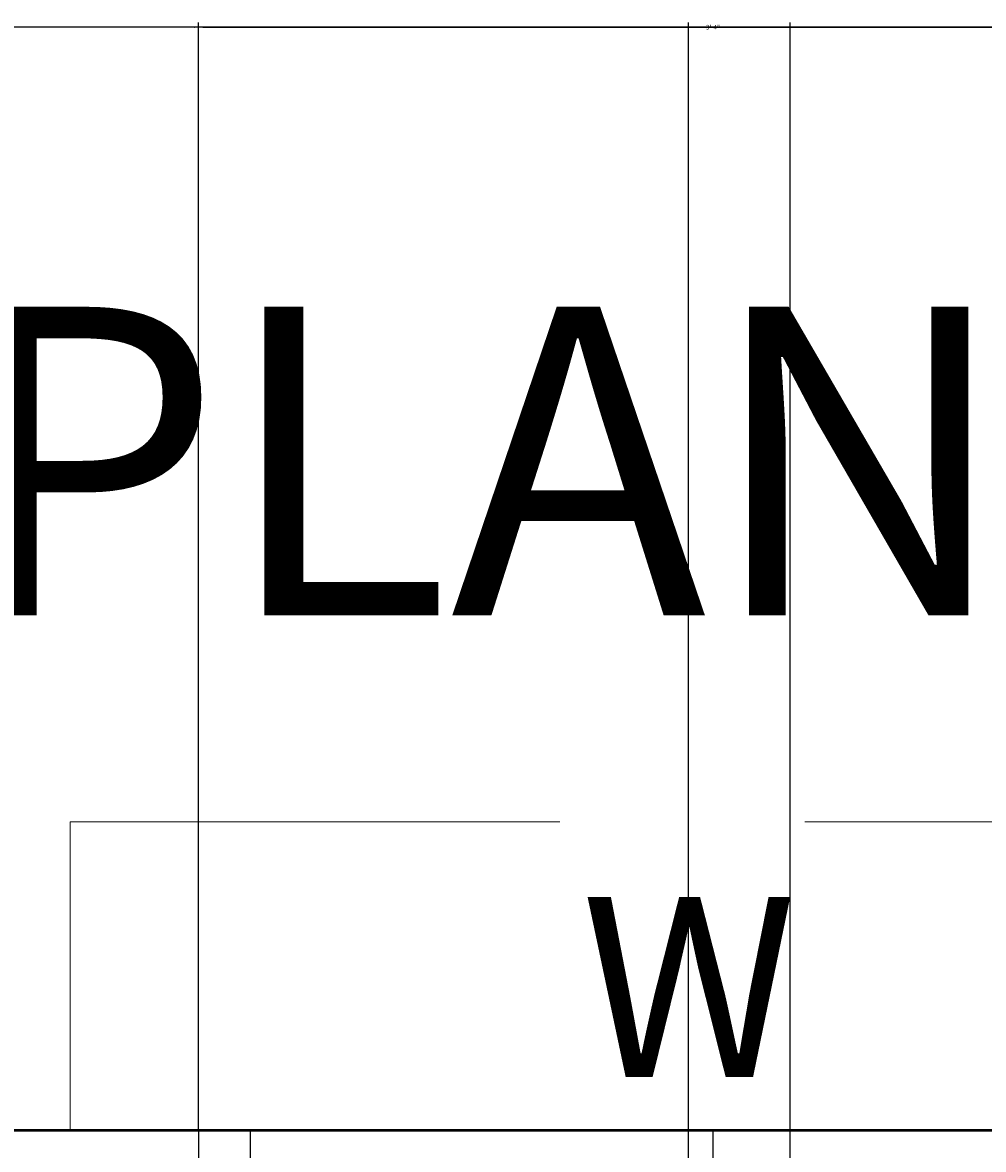
# Model space of a CAD drawing. Units: inches. Extents: x 37 to 824, y -700 to 234.
# Tile 74 of 77: x 332 to 370, y 190 to 234. Entities that reach past the tile are written whole.
import ezdxf

# ---------------------------------------------------------------- set-up
doc = ezdxf.new("R2010")
doc.units = ezdxf.units.IN
doc.header["$MEASUREMENT"] = 0
doc.linetypes.add('DASHED', pattern=[19.05, 12.7, -6.35])
for name, color, linetype, lineweight in [('A-ANNO-DIMS', 2, 'Continuous', 18), ('A-ANNO-TEXT', 7, 'Continuous', 18), ('A-GLAZ', 4, 'Continuous', 25), ('A-ROOF-OVHD', 1, 'DASHED', 18), ('A-WALL', 2, 'Continuous', 50)]:
    doc.layers.add(name, color=color, linetype=linetype, lineweight=lineweight)
doc.styles.get("Standard").update_dxf_attribs({"font": 'arial.ttf'})
doc.dimstyles.get("Standard").update_dxf_attribs({"dimtxt": 0.18, "dimasz": 0.18, "dimexe": 0.18, "dimexo": 0.0625, "dimgap": 0.09, "dimtad": 0, "dimtih": 1, "dimtoh": 1, "dimdec": 1, "dimzin": 0, "dimdsep": 46, "dimlunit": 4, "dimtxsty": 'Standard', "dimcen": 0.09, "dimadec": 0, "dimazin": 0, "dimtfac": 1, "dimtdec": 1, "dimtofl": 0, "dimtmove": 0, "dimatfit": 3, "dimfxl": 1, "dimtolj": 1, "dimtzin": 0, "dimarcsym": 0})

# ---------------------------------------------------------------- blocks, each defined once
blk = doc.blocks.new('WIN-900')
for p, q in [((0, 9), (0, 0)), ((2, 9), (2, 0)), ((20, 9), (20, 0)), ((38, 9), (38, 0)), ((40, 9), (40, 0)), ((38, 5.5), (2, 5.5)), ((38, 3.5), (2, 3.5))]:
    blk.add_line(p, q)
blk = doc.blocks.new('*D46')
at = {"layer": 'A-ANNO-DIMS', "color": 0, "lineweight": -2, "ltscale": 0.5, "transparency": 16777216}
for p, q in [((250.077, 191.153), (250.077, 234.17)), ((339.077, 191.153), (339.077, 234.17)), ((250.257, 233.99), (294.249, 233.99)), ((338.897, 233.99), (294.906, 233.99))]:
    blk.add_line(p, q, dxfattribs=at)
at = {"layer": 'A-ANNO-DIMS', "color": 0, "ltscale": 0.5, "transparency": 16777216}
for points in [[(250.257, 234.02), (250.257, 233.96), (250.077, 233.99)], [(338.897, 234.02), (338.897, 233.96), (339.077, 233.99)]]:
    blk.add_solid(points, dxfattribs=at)
at = {"layer": 'Defpoints', "color": 0, "ltscale": 0.5, "transparency": 16777216}
for p in [(339.077, 233.99), (250.077, 191.09), (339.077, 191.09)]:
    blk.add_point(p, dxfattribs=at)
at = {"layer": 'A-ANNO-DIMS', "color": 0, "ltscale": 0.5, "transparency": 16777216, "insert": (294.577, 233.99), "char_height": 0.18, "attachment_point": 5}
blk.add_mtext('\\A1;7\'-5"', dxfattribs=at)
blk = doc.blocks.new('*D47')
at = {"layer": 'A-ANNO-DIMS', "color": 0, "lineweight": -2, "ltscale": 0.5, "transparency": 16777216}
for p, q in [((339.077, 191.153), (339.077, 234.17)), ((379.077, 191.153), (379.077, 234.17)), ((339.257, 233.99), (358.748, 233.99)), ((378.897, 233.99), (359.406, 233.99))]:
    blk.add_line(p, q, dxfattribs=at)
at = {"layer": 'A-ANNO-DIMS', "color": 0, "ltscale": 0.5, "transparency": 16777216}
for points in [[(339.257, 234.02), (339.257, 233.96), (339.077, 233.99)], [(378.897, 234.02), (378.897, 233.96), (379.077, 233.99)]]:
    blk.add_solid(points, dxfattribs=at)
at = {"layer": 'Defpoints', "color": 0, "ltscale": 0.5, "transparency": 16777216}
for p in [(379.077, 233.99), (339.077, 191.09), (379.077, 191.09)]:
    blk.add_point(p, dxfattribs=at)
at = {"layer": 'A-ANNO-DIMS', "color": 0, "ltscale": 0.5, "transparency": 16777216, "insert": (359.077, 233.99), "char_height": 0.18, "attachment_point": 5}
blk.add_mtext('\\A1;3\'-4"', dxfattribs=at)
blk = doc.blocks.new('*D63')
at = {"layer": 'A-ANNO-DIMS', "color": 0, "lineweight": -2, "ltscale": 0.5, "transparency": 16777216}
for p, q in [((161.077, 191.153), (161.077, 234.17)), ((428.077, 191.153), (428.077, 234.17)), ((161.257, 233.99), (294.176, 233.99)), ((427.897, 233.99), (294.978, 233.99))]:
    blk.add_line(p, q, dxfattribs=at)
at = {"layer": 'A-ANNO-DIMS', "color": 0, "ltscale": 0.5, "transparency": 16777216}
for points in [[(161.257, 234.02), (161.257, 233.96), (161.077, 233.99)], [(427.897, 234.02), (427.897, 233.96), (428.077, 233.99)]]:
    blk.add_solid(points, dxfattribs=at)
at = {"layer": 'Defpoints', "color": 0, "ltscale": 0.5, "transparency": 16777216}
for p in [(428.077, 233.99), (161.077, 191.09), (428.077, 191.09)]:
    blk.add_point(p, dxfattribs=at)
at = {"layer": 'A-ANNO-DIMS', "color": 0, "ltscale": 0.5, "transparency": 16777216, "insert": (294.577, 233.99), "char_height": 0.18, "attachment_point": 5}
blk.add_mtext('\\A1;22\'-3"', dxfattribs=at)
blk = doc.blocks.new('*D78')
at = {"layer": 'A-ANNO-DIMS', "color": 0, "lineweight": -2, "ltscale": 0.5, "transparency": 16777216}
for p, q in [((290.077, 15.153), (290.077, 234.17)), ((362.077, 15.153), (362.077, 234.17)), ((290.257, 233.99), (325.747, 233.99)), ((361.897, 233.99), (326.407, 233.99))]:
    blk.add_line(p, q, dxfattribs=at)
at = {"layer": 'A-ANNO-DIMS', "color": 0, "ltscale": 0.5, "transparency": 16777216}
for points in [[(290.257, 234.02), (290.257, 233.96), (290.077, 233.99)], [(361.897, 234.02), (361.897, 233.96), (362.077, 233.99)]]:
    blk.add_solid(points, dxfattribs=at)
at = {"layer": 'Defpoints', "color": 0, "ltscale": 0.5, "transparency": 16777216}
for p in [(362.077, 233.99), (290.077, 15.09), (362.077, 15.09)]:
    blk.add_point(p, dxfattribs=at)
at = {"layer": 'A-ANNO-DIMS', "color": 0, "ltscale": 0.5, "transparency": 16777216, "insert": (326.077, 233.99), "char_height": 0.18, "attachment_point": 5}
blk.add_mtext('\\A1;6\'-0"', dxfattribs=at)
blk = doc.blocks.new('*D82')
at = {"layer": 'A-ANNO-DIMS', "color": 0, "lineweight": -2, "ltscale": 0.5, "transparency": 16777216}
for p, q in [((299.077, -206.847), (299.077, 234.17)), ((358.132, -206.847), (358.132, 234.17)), ((299.257, 233.99), (328.202, 233.99)), ((357.952, 233.99), (329.008, 233.99))]:
    blk.add_line(p, q, dxfattribs=at)
at = {"layer": 'A-ANNO-DIMS', "color": 0, "ltscale": 0.5, "transparency": 16777216}
for points in [[(299.257, 234.02), (299.257, 233.96), (299.077, 233.99)], [(357.952, 234.02), (357.952, 233.96), (358.132, 233.99)]]:
    blk.add_solid(points, dxfattribs=at)
at = {"layer": 'Defpoints', "color": 0, "ltscale": 0.5, "transparency": 16777216}
for p in [(358.132, 233.99), (299.077, -206.91), (358.132, -206.91)]:
    blk.add_point(p, dxfattribs=at)
at = {"layer": 'A-ANNO-DIMS', "color": 0, "ltscale": 0.5, "transparency": 16777216, "insert": (328.605, 233.99), "char_height": 0.18, "attachment_point": 5}
blk.add_mtext('\\A1;4\'-11"', dxfattribs=at)
blk = doc.blocks.new('*D83')
at = {"layer": 'A-ANNO-DIMS', "color": 0, "lineweight": -2, "ltscale": 0.5, "transparency": 16777216}
for p, q in [((358.132, -206.847), (358.132, 234.17)), ((419.077, -206.847), (419.077, 234.17)), ((358.312, 233.99), (388.275, 233.99)), ((418.897, 233.99), (388.934, 233.99))]:
    blk.add_line(p, q, dxfattribs=at)
at = {"layer": 'A-ANNO-DIMS', "color": 0, "ltscale": 0.5, "transparency": 16777216}
for points in [[(358.312, 234.02), (358.312, 233.96), (358.132, 233.99)], [(418.897, 234.02), (418.897, 233.96), (419.077, 233.99)]]:
    blk.add_solid(points, dxfattribs=at)
at = {"layer": 'Defpoints', "color": 0, "ltscale": 0.5, "transparency": 16777216}
for p in [(419.077, 233.99), (358.132, -206.91), (419.077, -206.91)]:
    blk.add_point(p, dxfattribs=at)
at = {"layer": 'A-ANNO-DIMS', "color": 0, "ltscale": 0.5, "transparency": 16777216, "insert": (388.605, 233.99), "char_height": 0.18, "attachment_point": 5}
blk.add_mtext('\\A1;5\'-1"', dxfattribs=at)

msp = doc.modelspace()

# ---------------------------------------------------------------- linework, layer by layer
at = {"layer": 'A-ROOF-OVHD', "ltscale": 1.5}
for p, q in [((334.077, 191.09), (334.077, 203.09)), ((334.077, 203.09), (384.077, 203.09)), ((339.077, 191.09), (334.077, 191.09))]:
    msp.add_line(p, q, dxfattribs=at)
at = {"layer": 'A-WALL'}
msp.add_line((299.077, 191.09), (428.077, 191.09), dxfattribs=at)

# ---------------------------------------------------------------- block references
at = {"layer": 'A-GLAZ'}
msp.add_blockref('WIN-900', (339.077, 182.09), dxfattribs=at)

# ---------------------------------------------------------------- texts
at = {"layer": 'A-ANNO-TEXT'}
for s, height, p in [('GROUND  FLOOR  PLAN', 12, (193.612, 211.117)), ('W', 7, (353.953, 193.168))]:
    msp.add_text(s, height=height, dxfattribs=at).set_placement(p)

# ---------------------------------------------------------------- dimensions: what is measured, and where the dimension line sits
at = {"layer": 'A-ANNO-DIMS', "ltscale": 0.5}
for base, p1, p2, picture, middle in [((428.077, 233.99), (161.077, 191.09), (428.077, 191.09), '*D63', (294.577, 233.99)), ((339.077, 233.99), (250.077, 191.09), (339.077, 191.09), '*D46', (294.577, 233.99)), ((362.077, 233.99), (290.077, 15.09), (362.077, 15.09), '*D78', (326.077, 233.99)), ((358.132, 233.99), (299.077, -206.91), (358.132, -206.91), '*D82', (328.605, 233.99)), ((379.077, 233.99), (339.077, 191.09), (379.077, 191.09), '*D47', (359.077, 233.99)), ((419.077, 233.99), (358.132, -206.91), (419.077, -206.91), '*D83', (388.605, 233.99))]:
    dim = msp.add_linear_dim(base=base, p1=p1, p2=p2, dimstyle='Standard', override={"dimdec": 1, "dimlfac": 1, "dimrnd": 0, "dimzin": 1, "dimdsep": 46, "dimlunit": 4, "dimfrac": 2}, dxfattribs=at)
    dim.commit()
    dim.dimension.update_dxf_attribs({"geometry": picture, "text_midpoint": middle})

doc.saveas('drawing.dxf')
